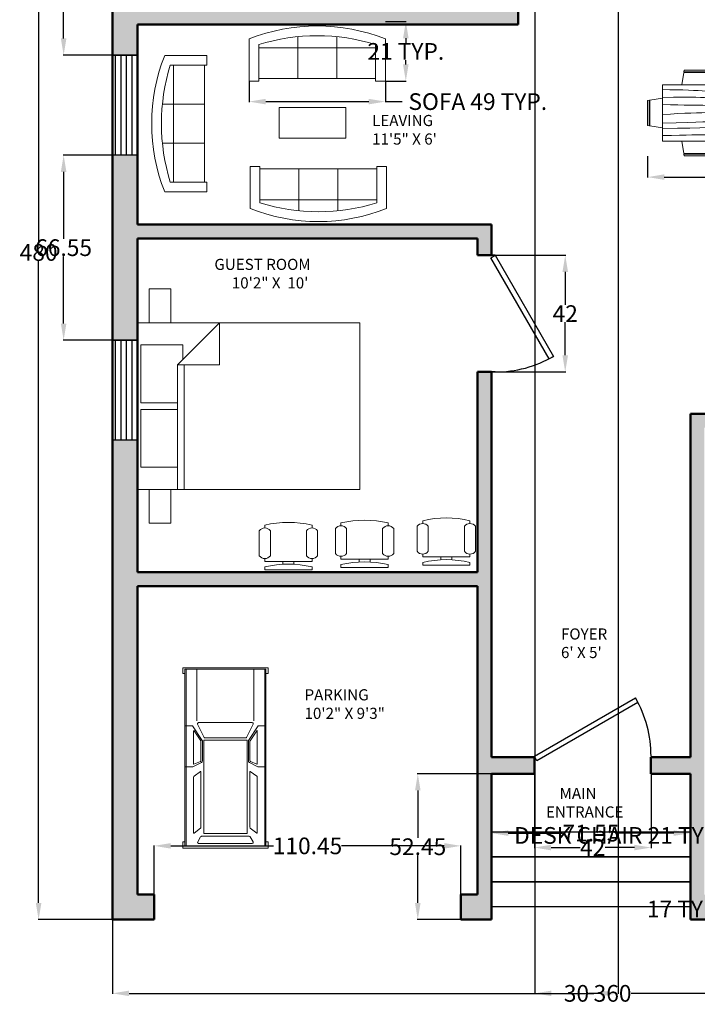
# Model space of a CAD drawing. Units: inches. Extents: x -40 to 482, y -490 to 102.
# Tile 1 of 4: x 2 to 245, y -490 to -136. Entities that reach past the tile are written whole.
import ezdxf

# ---------------------------------------------------------------- set-up
doc = ezdxf.new("R2010")
doc.units = ezdxf.units.IN
doc.header["$MEASUREMENT"] = 0
for name, color, linetype, lineweight in [('A-ANNO-DIMS', 2, 'Continuous', 18), ('A-ANNO-TEXT', 7, 'Continuous', 18), ('A-AREA-IDEN', 7, 'Continuous', 18), ('A-FLOR-PKNG', 8, 'Continuous', 13), ('A-FLOR-STRS', 7, 'Continuous', 25), ('A-FURN', 8, 'Continuous', 18), ('A-WALL', 7, 'Continuous', 50), ('A-WALL-PATT', 251, 'Continuous', 13), ('DOOR', 21, 'Continuous', 25), ('WINDOW', 151, 'Continuous', 25)]:
    doc.layers.add(name, color=color, linetype=linetype, lineweight=lineweight)
doc.styles.get("Standard").update_dxf_attribs({"font": 'arial.ttf'})
doc.dimstyles.get("Standard").update_dxf_attribs({"dimtxt": 6, "dimasz": 6, "dimexe": 0.18, "dimexo": 0.0625, "dimgap": 0.09, "dimtad": 0, "dimtih": 1, "dimtoh": 1, "dimdec": 3, "dimzin": 0, "dimdsep": 46, "dimlunit": 4, "dimtxsty": 'Standard', "dimcen": 0.09, "dimadec": 0, "dimazin": 0, "dimtfac": 1, "dimtdec": 3, "dimtofl": 0, "dimtmove": 0, "dimatfit": 3, "dimfxl": 1, "dimtolj": 1, "dimtzin": 0, "dimarcsym": 0})

# ---------------------------------------------------------------- blocks, each defined once
blk = doc.blocks.new('*U20')
for p, q in [((0, 0), (0, -6)), ((40, 0), (40, -6))]:
    blk.add_line(p, q)
blk.add_lwpolyline([(0, 0), (34.64, 20), (35.52, 18.48), (0.87, -1.52)], close=True)
blk.add_arc((0, 0), 40, 0, 30)
blk = doc.blocks.new('*U2')
for p, q in [((0, 0), (0, -6)), ((40, 0), (40, -6))]:
    blk.add_line(p, q)
blk.add_lwpolyline([(0, 0), (34.64, 20), (35.52, 18.48), (0.87, -1.52)], close=True)
blk.add_arc((0, 0), 40, 0, 30)
blk = doc.blocks.new('WINDOW')
for p, q in [((0, 0), (36, 0)), ((0, -9), (0, 0)), ((36, 0), (36, -9)), ((0, -2), (36, -2)), ((0, -4), (36, -4)), ((0, -6), (36, -6)), ((0, -8), (36, -8)), ((36, -9), (0, -9))]:
    blk.add_line(p, q)
blk = doc.blocks.new('Sofa - Roundback 7 ft.')
for p, q in [((-36.000027, -34), (-36.000027, -11.4696)), ((-12.00002, -32.4421), (-12.00003, -6.5971)), ((11.99997, -32.4421), (11.99998, -6.5971)), ((35.99998, -34), (35.99998, -11.4696)), ((-35.999844, -13.3819), (35.9998, -13.3819)), ((-36.000027, -32.4421), (35.99998, -32.4421))]:
    blk.add_line(p, q)
for points in [[(-36.000027, -34), (-42.000027, -34), (-42.000027, -8)], [(41.99998, -8), (41.99998, -34), (35.99998, -34)]]:
    blk.add_lwpolyline(points)
for centre, radius, start, end in [((0, -114.25), 114.25, 68.43141, 111.5686), ((-0.00001, -127.1968), 121.1968, 72.72033, 107.2797)]:
    blk.add_arc(centre, radius, start, end)
blk = doc.blocks.new('*U11')
for p, q in [((32, 987), (4462, 987)), ((32, 715), (1324, 715)), ((32, -715), (1324, -715)), ((32, -987), (4462, -987))]:
    blk.add_line(p, q)
for points in [[(141, 1016), (141, 1071), (0, 1071), (0, -1071), (141, -1071), (141, -1016), (32, -1016), (32, 1016)], [(32, 1016), (4462, 1016), (4462, -1016), (32, -1016)], [(4362, 1016), (4462, 1016), (4462, -1016), (4362, -1016), (4362, -1071), (4525, -1071), (4525, 1071), (4362, 1071)], [(1815, 546), (4151, 546), (4151, -546), (1815, -546)]]:
    blk.add_lwpolyline(points, close=True)
for points in [[(1451, 1016), (1451, 823), (1822, 580, 0.086577), (1843, 576), (2326, 576, 0.227875), (2376, 600), (2482, 816), (2482, 1016)], [(1451, -1016), (1451, -823), (1822, -580, -0.086577), (1843, -576), (2326, -576, -0.227875), (2376, -600), (2482, -816), (2482, -1016)]]:
    blk.add_lwpolyline(points, format="xyb")
for points in [[(1577, 786), (1832, 618, 0.146139), (1846, 614), (2322, 614, 0.29766), (2345, 629), (2415, 789, 0.541236), (2409, 798), (1580, 798, 0.744989)], [(2596, 624), (2717, 787, -0.236929), (2737, 798), (4138, 798, -0.621576), (4143, 787), (4018, 624, -0.233368), (3998, 614), (2601, 614, -0.616908)], [(1410, 697), (1742, 531, -0.284287), (1756, 508), (1756, -508, -0.284287), (1742, -531), (1410, -697, -0.557284), (1373, -674), (1373, 674, -0.557284)], [(4366, 694), (4237, 622, 0.271143), (4224, 599), (4224, -599, 0.271143), (4237, -622), (4366, -694, 0.573387), (4404, -672), (4404, 672, 0.573387)], [(1577, -786), (1832, -618, -0.146139), (1846, -614), (2322, -614, -0.29766), (2345, -629), (2415, -789, -0.541236), (2409, -798), (1580, -798, -0.744989)], [(2596, -624), (2717, -787, 0.236929), (2737, -798), (4138, -798, 0.621576), (4143, -787), (4018, -624, 0.233368), (3998, -614), (2601, -614, 0.616908)]]:
    blk.add_lwpolyline(points, format="xyb", close=True)
blk = doc.blocks.new('Bed - Queen')
for p, q in [((0, -80.00003), (0, 0)), ((0, 0), (59.99999, 0)), ((59.99999, 0), (59.99999, -80.00003)), ((7.99999, -1.2), (28.79998, -1.2)), ((7.99999, -14.4), (7.99999, -1.2)), ((28.79998, -1.2), (28.79998, -14.4)), ((31.19999, -1.2), (51.99999, -1.2)), ((31.19999, -14.4), (31.19999, -1.2)), ((51.99999, -1.2), (51.99999, -16.4)), ((0, -14.4), (44.8, -14.4)), ((44.8, -16.8), (0, -16.8)), ((59.99999, -29.6), (44.8, -14.4)), ((44.8, -14.4), (44.8, -29.6)), ((51.99999, -16.4), (46.79936, -16.4)), ((44.8, -29.6), (59.99999, -29.6)), ((59.99999, -80.00003), (0, -80.00003))]:
    blk.add_line(p, q)
blk = doc.blocks.new('Chair - Desk')
for p, q in [((-8.5, 0), (-8.5, -1)), ((-8.5, 0), (8.5, 0)), ((8.5, 0), (8.5, -1)), ((-8.5, -3), (-8.5, -4)), ((-8.5, -3), (8.5, -3)), ((-2, -3), (-2, -1.9355)), ((2, -1.9576), (2, -3)), ((8.5, -3), (8.5, -4)), ((-10.5, -5), (-10.5, -14)), ((-6.5, -14), (-6.5, -5)), ((6.5, -5), (6.5, -14)), ((10.5, -14), (10.5, -5)), ((-8.5, -15), (-8.5, -16)), ((8.5, -15), (8.5, -16))]:
    blk.add_line(p, q)
for centre, radius, start, end in [((0, 34.625), 36.625, 256.5803, 283.4197), ((-8.5, -6.5), 2.5, 36.8699, 143.1301), ((8.5, -6.5), 2.5, 36.8699, 143.1301), ((-8.5, -12.5), 2.5, 216.8699, 323.1301), ((8.5, -12.5), 2.5, 216.8699, 323.1301), ((0, 19.625), 36.625, 256.5803, 283.4197)]:
    blk.add_arc(centre, radius, start, end)
blk = doc.blocks.new('Dining Set - 36 x 72 in.')
for p, q in [((-22.2343, 26.00059), (-23.4847, 17.99762)), ((-22.2304, 26), (-5.7608, 26)), ((-22, 27.5), (-22.1562, 26.50042)), ((-5.8416, 26.5), (-22.1534, 26.5)), ((-22, 27.5), (-6, 27.5)), ((-5.8437, 26.49966), (-6, 27.5)), ((-4.5152, 17.99762), (-5.7655, 25.99926)), ((5.7657, 26.00059), (4.5153, 17.99762)), ((5.7696, 26), (22.2392, 26)), ((6, 27.5), (5.8438, 26.50042)), ((22.1584, 26.5), (5.8466, 26.5)), ((6, 27.5), (22, 27.5)), ((22.1563, 26.49966), (22, 27.5)), ((23.4848, 17.99762), (22.2345, 25.99926)), ((36, 18), (-36, 18)), ((-36, 18), (-36, -18)), ((36, -18), (36, 18)), ((-45.5, 8), (-44.5004, 8.15617)), ((-45.5, 8), (-45.5, -8)), ((-44.5, -8.15843), (-44.5, 8.15338)), ((-44.0006, 8.23428), (-35.9976, 9.48474)), ((-44, 8.23041), (-44, -8.23915)), ((44.0006, 8.23428), (35.9976, 9.48474)), ((44, 8.23041), (44, -8.23915)), ((44.5, -8.15843), (44.5, 8.15338)), ((45.5, 8), (44.5005, 8.15617)), ((45.5, 8), (45.5, -8)), ((-44.4997, -8.15631), (-45.5, -8)), ((-35.9976, -9.48476), (-43.9993, -8.2345)), ((35.9976, -9.48476), (43.9993, -8.2345)), ((44.4997, -8.15631), (45.5, -8)), ((-36, -18), (36, -18)), ((-22.2343, -26.0006), (-23.4847, -17.99762)), ((-4.5152, -17.99762), (-5.7655, -25.99928)), ((5.7657, -26.0006), (4.5153, -17.99762)), ((23.4848, -17.99762), (22.2345, -25.99928)), ((-22.2304, -26), (-5.7608, -26)), ((-22, -27.5), (-22.1562, -26.50044)), ((-5.8416, -26.5), (-22.1534, -26.5)), ((-22, -27.5), (-6, -27.5)), ((-5.8437, -26.49967), (-6, -27.5)), ((5.7696, -26), (22.2392, -26)), ((6, -27.5), (5.8438, -26.50044)), ((22.1584, -26.5), (5.8466, -26.5)), ((6, -27.5), (22, -27.5)), ((22.1563, -26.49967), (22, -27.5))]:
    blk.add_line(p, q)
for points in [[(-36, 15), (-31.1772, 14.97754), (-26.8079, 14.91406), (-22.8538, 14.81543), (-19.276, 14.6875), (-16.0362, 14.53613), (-13.0957, 14.36718), (-10.4159, 14.18652), (-7.9583, 14), (-5.6904, 13.81315), (-3.6035, 13.63021), (-1.6954, 13.45508), (0.0365, 13.29166), (1.5945, 13.14388), (2.9811, 13.01562), (4.1988, 12.9108), (5.25, 12.83333), (6.1393, 12.78613), (6.8802, 12.76823), (7.4883, 12.77767), (7.9792, 12.8125), (8.3685, 12.87077), (8.6719, 12.95052), (8.9049, 13.0498), (9.0833, 13.16666), (9.2205, 13.29899), (9.3216, 13.44401), (9.3895, 13.59879), (9.4271, 13.76041), (9.4373, 13.92594), (9.4232, 14.09245), (9.3875, 14.257), (9.3333, 14.41666), (9.2638, 14.56917), (9.1836, 14.71484), (9.0975, 14.85465), (9.0104, 14.98958), (8.9272, 15.1206), (8.8529, 15.2487), (8.7922, 15.37483), (8.75, 15.5), (8.7305, 15.62467), (8.7344, 15.74739), (8.7617, 15.86621), (8.8125, 15.97916), (8.8867, 16.08431), (8.9844, 16.17968), (9.1055, 16.26334), (9.25, 16.33333), (9.4189, 16.38802), (9.6172, 16.42708), (9.8506, 16.45052), (10.125, 16.45833), (10.4463, 16.45052), (10.8203, 16.42708), (11.2529, 16.38802), (11.75, 16.33333), (12.3184, 16.26318), (12.9694, 16.17838), (13.7151, 16.07991), (14.5677, 15.96875), (15.5395, 15.84586), (16.6426, 15.71224), (17.8893, 15.56884), (19.2917, 15.41666), (20.859, 15.25667), (22.5879, 15.08984), (24.4721, 14.91715), (26.5052, 14.73958), (28.6809, 14.5581), (30.9929, 14.3737), (33.4347, 14.18733), (36, 14)], [(-36, 10), (-28.9766, 10.14274), (-23.1725, 10.20442), (-18.4241, 10.19775), (-14.5677, 10.13541), (-11.4399, 10.03011), (-8.877, 9.89453), (-6.7154, 9.74137), (-4.7917, 9.58333), (-2.9698, 9.43082), (-1.2246, 9.28515), (0.4415, 9.14534), (2.026, 9.01041), (3.5266, 8.87939), (4.9408, 8.7513), (6.266, 8.62516), (7.5, 8.5), (8.6411, 8.37549), (9.6914, 8.2539), (10.6538, 8.13818), (11.5312, 8.03125), (12.3267, 7.93603), (13.043, 7.85547), (13.6831, 7.79248), (14.25, 7.75), (14.7471, 7.7303), (15.1797, 7.73307), (15.5537, 7.75732), (15.875, 7.80208), (16.1494, 7.86637), (16.3828, 7.94922), (16.5811, 8.04964), (16.75, 8.16666), (16.8944, 8.29915), (17.0143, 8.44531), (17.1089, 8.60319), (17.1771, 8.77083), (17.218, 8.94629), (17.2305, 9.1276), (17.2137, 9.31282), (17.1667, 9.5), (17.0895, 9.6875), (16.987, 9.875), (16.8649, 10.0625), (16.7292, 10.25), (16.5856, 10.4375), (16.4401, 10.625), (16.2985, 10.8125), (16.1667, 11), (16.05, 11.18733), (15.9518, 11.3737), (15.8752, 11.5581), (15.8229, 11.73958), (15.798, 11.91715), (15.8034, 12.08984), (15.842, 12.25667), (15.9167, 12.41666), (16.0295, 12.56836), (16.1784, 12.70833), (16.3605, 12.83268), (16.5729, 12.9375), (16.8127, 13.01888), (17.0768, 13.07291), (17.3625, 13.0957), (17.6667, 13.08333), (17.9894, 13.03312), (18.3418, 12.94726), (18.7382, 12.82918), (19.1927, 12.68229), (19.7195, 12.51001), (20.3327, 12.31575), (21.0465, 12.10294), (21.875, 11.875), (22.8357, 11.63354), (23.959, 11.37304), (25.2786, 11.08618), (26.8282, 10.76562), (28.6414, 10.40405), (30.752, 9.99414), (33.1936, 9.52856), (36, 9)], [(-36, 5.5), (-30.7157, 5.3348), (-26.069, 5.20963), (-21.9946, 5.11767), (-18.4271, 5.05208), (-15.3009, 5.00602), (-12.5508, 4.97265), (-10.1112, 4.94515), (-7.9167, 4.91666), (-5.909, 4.88167), (-4.0586, 4.83984), (-2.3429, 4.79215), (-0.7396, 4.73958), (0.7739, 4.6831), (2.22, 4.6237), (3.6213, 4.56233), (5, 4.5), (6.373, 4.43782), (7.7344, 4.3776), (9.0723, 4.32129), (10.375, 4.27083), (11.6309, 4.22819), (12.8281, 4.19531), (13.9551, 4.17415), (15, 4.16666), (15.954, 4.17448), (16.819, 4.19791), (17.6001, 4.23698), (18.3021, 4.29166), (18.9299, 4.36198), (19.4883, 4.44791), (19.9823, 4.54948), (20.4167, 4.66666), (20.7969, 4.79899), (21.1302, 4.94401), (21.4245, 5.09879), (21.6875, 5.26041), (21.9271, 5.42594), (22.1511, 5.59245), (22.3672, 5.757), (22.5834, 5.91666), (22.8065, 6.06868), (23.0404, 6.21093), (23.2879, 6.34147), (23.5521, 6.45833), (23.8358, 6.55957), (24.142, 6.64323), (24.4735, 6.70735), (24.8334, 6.75), (25.2235, 6.76969), (25.642, 6.76692), (26.0858, 6.74267), (26.5521, 6.69791), (27.0379, 6.63362), (27.5404, 6.55078), (28.0565, 6.45036), (28.5834, 6.33333), (29.1242, 6.19987), (29.7071, 6.04687), (30.3661, 5.87044), (31.1354, 5.66666), (32.0493, 5.43164), (33.142, 5.16146), (34.4475, 4.85221), (36, 4.5)], [(-36, -1), (-30.7915, -0.6591), (-26.0195, -0.38216), (-21.6519, -0.16284), (-17.6563, 0.00521), (-14.0005, 0.12833), (-10.6523, 0.21289), (-7.5796, 0.26522), (-4.75, 0.29166), (-2.134, 0.29793), (0.2878, 0.28711), (2.5317, 0.26163), (4.6146, 0.22396), (6.5529, 0.17651), (8.3633, 0.12174), (10.0623, 0.06209), (11.6667, 0), (13.1899, -0.06201), (14.6341, -0.1211), (15.9982, -0.17432), (17.2813, -0.21875), (18.4823, -0.25147), (19.6003, -0.26953), (20.6343, -0.27002), (21.5834, -0.25), (22.4481, -0.20768), (23.2357, -0.14584), (23.9549, -0.06836), (24.6146, 0.02083), (25.2235, 0.11784), (25.7904, 0.21875), (26.3241, 0.31966), (26.8334, 0.41666), (27.3265, 0.50618), (27.8099, 0.58593), (28.2894, 0.65397), (28.7709, 0.70833), (29.2601, 0.74707), (29.763, 0.76823), (30.2855, 0.76985), (30.8334, 0.75), (31.4088, 0.70784), (31.9994, 0.64713), (32.589, 0.57275), (33.1615, 0.48958), (33.7008, 0.4025), (34.1908, 0.3164), (34.6153, 0.23616), (34.9584, 0.16666), (35.2099, 0.11165), (35.3848, 0.07031), (35.504, 0.04069), (35.5886, 0.02083), (35.6594, 0.00879), (35.7377, 0.0026), (35.8442, 0.00032), (36, 0)], [(-36, -6.5), (-27.1843, -6.31267), (-20.084, -6.1263), (-14.469, -5.9419), (-10.1094, -5.76042), (-6.7752, -5.58285), (-4.2363, -5.41016), (-2.2629, -5.24333), (-0.625, -5.08334), (0.8708, -4.93099), (2.2715, -4.78646), (3.5872, -4.64974), (4.8281, -4.52084), (6.0046, -4.39974), (7.127, -4.28646), (8.2053, -4.18099), (9.25, -4.08334), (10.2705, -3.99382), (11.2734, -3.91407), (12.2647, -3.84603), (13.25, -3.79167), (14.2354, -3.75293), (15.2266, -3.73177), (16.2295, -3.73015), (17.25, -3.75), (18.2912, -3.79248), (19.3451, -3.85547), (20.4009, -3.93604), (21.4479, -4.03125), (22.4754, -4.13819), (23.4727, -4.25391), (24.4289, -4.37549), (25.3334, -4.5), (26.1785, -4.62492), (26.9694, -4.74935), (27.7145, -4.87281), (28.4219, -4.99479), (29.1, -5.11483), (29.7572, -5.23242), (30.4016, -5.34709), (31.0417, -5.45834), (31.6837, -5.56437), (32.3262, -5.65821), (32.9658, -5.73153), (33.599, -5.77604), (34.2224, -5.78345), (34.8327, -5.74545), (35.4264, -5.65373), (36, -5.5)], [(-36, -10), (-26.4022, -9.81299), (-18.4675, -9.62891), (-11.9839, -9.45069), (-6.7396, -9.28125), (-2.5226, -9.12354), (0.8789, -8.98047), (3.6769, -8.85498), (6.0833, -8.75), (8.2767, -8.66765), (10.3021, -8.60677), (12.1712, -8.56543), (13.8958, -8.54167), (15.4876, -8.53353), (16.9583, -8.53907), (18.3197, -8.55632), (19.5834, -8.58334), (20.7616, -8.61841), (21.8685, -8.66081), (22.9188, -8.71004), (23.9271, -8.76563), (24.9081, -8.82707), (25.8763, -8.89388), (26.8465, -8.96558), (27.8334, -9.04167), (28.8474, -9.12118), (29.8828, -9.20117), (30.93, -9.27824), (31.9792, -9.34896), (33.0205, -9.40991), (34.0443, -9.45768), (35.0407, -9.48885), (36, -9.5)], [(-36, -14.5), (-30.0881, -14.33513), (-25.0332, -14.21224), (-20.7312, -14.12647), (-17.0781, -14.07292), (-13.97, -14.04671), (-11.3027, -14.04297), (-8.9724, -14.05681), (-6.875, -14.08334), (-4.9224, -14.11833), (-3.0905, -14.16016), (-1.3709, -14.20785), (0.2448, -14.26042), (1.7647, -14.3169), (3.1973, -14.3763), (4.5507, -14.43767), (5.8333, -14.5), (7.0554, -14.5621), (8.235, -14.62175), (9.3922, -14.67652), (10.5469, -14.72396), (11.7192, -14.76164), (12.929, -14.78711), (14.1965, -14.79794), (15.5417, -14.79167), (16.9933, -14.76424), (18.6152, -14.70508), (20.4804, -14.60197), (22.6615, -14.44271), (25.2312, -14.21509), (28.2624, -13.9069), (31.8277, -13.50594), (36, -13)]]:
    blk.add_lwpolyline(points)
blk = doc.blocks.new('NIGHTSTAND')
blk.add_lwpolyline([(0, 12.15), (7.78, 12.15), (7.78, 0), (0, 0)], close=True)
blk = doc.blocks.new('*D28')
at = {"layer": 'A-ANNO-DIMS', "color": 0, "lineweight": -2, "transparency": 16777216}
for p, q in [((264.6, -429.23), (258.6, -429.23)), ((264.6, -432.32), (264.6, -429.05)), ((279.6, -429.23), (270.6, -429.23)), ((285.6, -432.32), (285.6, -429.05))]:
    blk.add_line(p, q, dxfattribs=at)
at = {"layer": 'A-ANNO-DIMS', "color": 0, "transparency": 16777216}
for points in [[(270.6, -428.23), (270.6, -430.23), (264.6, -429.23)], [(279.6, -428.23), (279.6, -430.23), (285.6, -429.23)]]:
    blk.add_solid(points, dxfattribs=at)
at = {"layer": 'Defpoints', "color": 0, "transparency": 16777216}
for p in [(264.6, -429.23), (264.6, -432.38), (285.6, -432.38)]:
    blk.add_point(p, dxfattribs=at)
at = {"layer": 'A-ANNO-DIMS', "color": 0, "transparency": 16777216, "insert": (217.27, -429.23), "char_height": 6, "attachment_point": 5}
blk.add_mtext('\\A1;DESK CHAIR 21 TYP.', dxfattribs=at)
blk = doc.blocks.new('*D29')
at = {"layer": 'A-ANNO-DIMS', "color": 0, "lineweight": -2, "transparency": 16777216}
for p, q in [((264.53, -432.38), (261.27, -432.38)), ((261.45, -438.38), (261.45, -443.71)), ((264.53, -449.71), (261.27, -449.71)), ((261.45, -449.71), (261.45, -455.71)), ((261.45, -455.71), (255.45, -455.71))]:
    blk.add_line(p, q, dxfattribs=at)
at = {"layer": 'A-ANNO-DIMS', "color": 0, "transparency": 16777216}
for points in [[(260.45, -438.38), (262.45, -438.38), (261.45, -432.38)], [(260.45, -443.71), (262.45, -443.71), (261.45, -449.71)]]:
    blk.add_solid(points, dxfattribs=at)
at = {"layer": 'Defpoints', "color": 0, "transparency": 16777216}
for p in [(264.6, -432.38), (261.45, -449.71), (264.6, -449.71)]:
    blk.add_point(p, dxfattribs=at)
at = {"layer": 'A-ANNO-DIMS', "color": 0, "transparency": 16777216, "insert": (241.04, -455.71), "char_height": 6, "attachment_point": 5}
blk.add_mtext('\\A1;17 TYP.', dxfattribs=at)
blk = doc.blocks.new('*D34')
at = {"layer": 'A-ANNO-DIMS', "color": 0, "lineweight": -2, "transparency": 16777216}
for p, q in [((84.04, -157.95), (84.04, -165.42)), ((133.1, -157.95), (133.1, -165.42)), ((90.04, -165.24), (127.1, -165.24)), ((133.1, -165.24), (139.1, -165.24))]:
    blk.add_line(p, q, dxfattribs=at)
at = {"layer": 'A-ANNO-DIMS', "color": 0, "transparency": 16777216}
for points in [[(90.04, -164.24), (90.04, -166.24), (84.04, -165.24)], [(127.1, -164.24), (127.1, -166.24), (133.1, -165.24)]]:
    blk.add_solid(points, dxfattribs=at)
at = {"layer": 'Defpoints', "color": 0, "transparency": 16777216}
for p in [(84.04, -157.88), (133.1, -157.88), (133.1, -165.24)]:
    blk.add_point(p, dxfattribs=at)
at = {"layer": 'A-ANNO-DIMS', "color": 0, "transparency": 16777216, "insert": (166.36, -165.24), "char_height": 6, "attachment_point": 5}
blk.add_mtext('\\A1;SOFA 49 TYP.', dxfattribs=at)
blk = doc.blocks.new('*D35')
at = {"layer": 'A-ANNO-DIMS', "color": 0, "lineweight": -2, "transparency": 16777216}
for p, q in [((133.17, -136.47), (140.64, -136.47)), ((140.46, -142.47), (140.46, -144.07)), ((140.46, -151.88), (140.46, -150.28)), ((133.17, -157.88), (140.64, -157.88))]:
    blk.add_line(p, q, dxfattribs=at)
at = {"layer": 'A-ANNO-DIMS', "color": 0, "transparency": 16777216}
for points in [[(139.46, -142.47), (141.46, -142.47), (140.46, -136.47)], [(139.46, -151.88), (141.46, -151.88), (140.46, -157.88)]]:
    blk.add_solid(points, dxfattribs=at)
at = {"layer": 'Defpoints', "color": 0, "transparency": 16777216}
for p in [(133.1, -136.47), (140.46, -136.47), (133.1, -157.88)]:
    blk.add_point(p, dxfattribs=at)
at = {"layer": 'A-ANNO-DIMS', "color": 0, "transparency": 16777216, "insert": (140.46, -147.18), "char_height": 6, "attachment_point": 5}
blk.add_mtext('\\A1;21 TYP.', dxfattribs=at)
blk = doc.blocks.new('*D50')
at = {"layer": 'A-ANNO-DIMS', "color": 0, "lineweight": -2, "transparency": 16777216}
for p, q in [((227.47, -184.82), (227.47, -192.58)), ((278.45, -184.82), (278.45, -192.58)), ((233.47, -192.4), (272.45, -192.4)), ((278.45, -192.4), (284.45, -192.4))]:
    blk.add_line(p, q, dxfattribs=at)
at = {"layer": 'A-ANNO-DIMS', "color": 0, "transparency": 16777216}
for points in [[(233.47, -191.4), (233.47, -193.4), (227.47, -192.4)], [(272.45, -191.4), (272.45, -193.4), (278.45, -192.4)]]:
    blk.add_solid(points, dxfattribs=at)
at = {"layer": 'Defpoints', "color": 0, "transparency": 16777216}
for p in [(227.47, -184.75), (278.45, -184.75), (278.45, -192.4)]:
    blk.add_point(p, dxfattribs=at)
at = {"layer": 'A-ANNO-DIMS', "color": 0, "transparency": 16777216, "insert": (313.26, -192.4), "char_height": 6, "attachment_point": 5}
blk.add_mtext('\\A1;DINING SET 51', dxfattribs=at)
blk = doc.blocks.new('*D52')
at = {"layer": 'A-ANNO-DIMS', "color": 0, "lineweight": -2, "transparency": 16777216}
for p, q in [((34.86, -459.57), (34.86, -486.22)), ((394.86, -459.57), (394.86, -486.22)), ((40.86, -486.04), (208.15, -486.04)), ((388.86, -486.04), (221.56, -486.04))]:
    blk.add_line(p, q, dxfattribs=at)
at = {"layer": 'A-ANNO-DIMS', "color": 0, "transparency": 16777216}
for points in [[(40.86, -485.04), (40.86, -487.04), (34.86, -486.04)], [(388.86, -485.04), (388.86, -487.04), (394.86, -486.04)]]:
    blk.add_solid(points, dxfattribs=at)
at = {"layer": 'Defpoints', "color": 0, "transparency": 16777216}
for p in [(34.86, -459.51), (394.86, -459.51), (394.86, -486.04)]:
    blk.add_point(p, dxfattribs=at)
at = {"layer": 'A-ANNO-DIMS', "color": 0, "transparency": 16777216, "insert": (214.86, -486.04), "char_height": 6, "attachment_point": 5}
blk.add_mtext('\\A1;360', dxfattribs=at)
blk = doc.blocks.new('*D53')
at = {"layer": 'A-ANNO-DIMS', "color": 0, "lineweight": -2, "transparency": 16777216}
for p, q in [((34.79, 20.49), (8.14, 20.49)), ((8.32, 14.49), (8.32, -216.36)), ((8.32, -453.51), (8.32, -222.66)), ((34.79, -459.51), (8.14, -459.51))]:
    blk.add_line(p, q, dxfattribs=at)
at = {"layer": 'A-ANNO-DIMS', "color": 0, "transparency": 16777216}
for points in [[(7.32, 14.49), (9.32, 14.49), (8.32, 20.49)], [(7.32, -453.51), (9.32, -453.51), (8.32, -459.51)]]:
    blk.add_solid(points, dxfattribs=at)
at = {"layer": 'Defpoints', "color": 0, "transparency": 16777216}
for p in [(8.32, 20.49), (34.86, 20.49), (34.86, -459.51)]:
    blk.add_point(p, dxfattribs=at)
at = {"layer": 'A-ANNO-DIMS', "color": 0, "transparency": 16777216, "insert": (8.32, -219.51), "char_height": 6, "attachment_point": 5}
blk.add_mtext('\\A1;480', dxfattribs=at)
blk = doc.blocks.new('*D57')
at = {"layer": 'A-ANNO-DIMS', "color": 0, "lineweight": -2, "transparency": 16777216}
for p, q in [((43.79, -76.86), (17.14, -76.86)), ((17.32, -82.86), (17.32, -109.54)), ((17.32, -142.52), (17.32, -115.84)), ((43.79, -148.52), (17.14, -148.52))]:
    blk.add_line(p, q, dxfattribs=at)
at = {"layer": 'A-ANNO-DIMS', "color": 0, "transparency": 16777216}
for points in [[(16.32, -82.86), (18.32, -82.86), (17.32, -76.86)], [(16.32, -142.52), (18.32, -142.52), (17.32, -148.52)]]:
    blk.add_solid(points, dxfattribs=at)
at = {"layer": 'Defpoints', "color": 0, "transparency": 16777216}
for p in [(17.32, -76.86), (43.86, -76.86), (43.86, -148.52)]:
    blk.add_point(p, dxfattribs=at)
at = {"layer": 'A-ANNO-DIMS', "color": 0, "transparency": 16777216, "insert": (17.32, -112.69), "char_height": 6, "attachment_point": 5}
blk.add_mtext('\\A1;71.66', dxfattribs=at)
blk = doc.blocks.new('*D58')
at = {"layer": 'A-ANNO-DIMS', "color": 0, "lineweight": -2, "transparency": 16777216}
for p, q in [((43.79, -184.52), (17.14, -184.52)), ((17.32, -190.52), (17.32, -214.64)), ((17.32, -245.07), (17.32, -220.95)), ((43.79, -251.07), (17.14, -251.07))]:
    blk.add_line(p, q, dxfattribs=at)
at = {"layer": 'A-ANNO-DIMS', "color": 0, "transparency": 16777216}
for points in [[(16.32, -190.52), (18.32, -190.52), (17.32, -184.52)], [(16.32, -245.07), (18.32, -245.07), (17.32, -251.07)]]:
    blk.add_solid(points, dxfattribs=at)
at = {"layer": 'Defpoints', "color": 0, "transparency": 16777216}
for p in [(17.32, -184.52), (43.86, -184.52), (43.86, -251.07)]:
    blk.add_point(p, dxfattribs=at)
at = {"layer": 'A-ANNO-DIMS', "color": 0, "transparency": 16777216, "insert": (17.32, -217.79), "char_height": 6, "attachment_point": 5}
blk.add_mtext('\\A1;66.55', dxfattribs=at)
blk = doc.blocks.new('*D63')
at = {"layer": 'A-ANNO-DIMS', "color": 0, "lineweight": -2, "transparency": 16777216}
for p, q in [((186.86, -53.57), (186.86, -486.22)), ((216.86, -53.57), (216.86, -486.22)), ((192.86, -486.04), (197.48, -486.04)), ((210.86, -486.04), (206.23, -486.04))]:
    blk.add_line(p, q, dxfattribs=at)
at = {"layer": 'A-ANNO-DIMS', "color": 0, "transparency": 16777216}
for points in [[(192.86, -485.04), (192.86, -487.04), (186.86, -486.04)], [(210.86, -485.04), (210.86, -487.04), (216.86, -486.04)]]:
    blk.add_solid(points, dxfattribs=at)
at = {"layer": 'Defpoints', "color": 0, "transparency": 16777216}
for p in [(186.86, -53.51), (216.86, -53.51), (216.86, -486.04)]:
    blk.add_point(p, dxfattribs=at)
at = {"layer": 'A-ANNO-DIMS', "color": 0, "transparency": 16777216, "insert": (201.86, -486.04), "char_height": 6, "attachment_point": 5}
blk.add_mtext('\\A1;30', dxfattribs=at)
blk = doc.blocks.new('*D65')
at = {"layer": 'A-ANNO-DIMS', "color": 0, "lineweight": -2, "transparency": 16777216}
for p, q in [((171.36, -220.51), (198.01, -220.51)), ((197.83, -226.51), (197.83, -238.41)), ((197.83, -256.51), (197.83, -244.61)), ((171.36, -262.51), (198.01, -262.51))]:
    blk.add_line(p, q, dxfattribs=at)
at = {"layer": 'A-ANNO-DIMS', "color": 0, "transparency": 16777216}
for points in [[(196.83, -226.51), (198.83, -226.51), (197.83, -220.51)], [(196.83, -256.51), (198.83, -256.51), (197.83, -262.51)]]:
    blk.add_solid(points, dxfattribs=at)
at = {"layer": 'Defpoints', "color": 0, "transparency": 16777216}
for p in [(171.3, -220.51), (171.3, -262.51), (197.83, -262.51)]:
    blk.add_point(p, dxfattribs=at)
at = {"layer": 'A-ANNO-DIMS', "color": 0, "transparency": 16777216, "insert": (197.83, -241.51), "char_height": 6, "attachment_point": 5}
blk.add_mtext('\\A1;42', dxfattribs=at)
blk = doc.blocks.new('*D71')
at = {"layer": 'A-ANNO-DIMS', "color": 0, "lineweight": -2, "transparency": 16777216}
for p, q in [((49.86, -459.45), (49.86, -432.8)), ((55.86, -432.98), (92.79, -432.98)), ((154.3, -432.98), (117.36, -432.98)), ((160.3, -459.45), (160.3, -432.8))]:
    blk.add_line(p, q, dxfattribs=at)
at = {"layer": 'A-ANNO-DIMS', "color": 0, "transparency": 16777216}
for points in [[(55.86, -431.98), (55.86, -433.98), (49.86, -432.98)], [(154.3, -431.98), (154.3, -433.98), (160.3, -432.98)]]:
    blk.add_solid(points, dxfattribs=at)
at = {"layer": 'Defpoints', "color": 0, "transparency": 16777216}
for p in [(160.3, -432.98), (49.86, -459.51), (160.3, -459.51)]:
    blk.add_point(p, dxfattribs=at)
at = {"layer": 'A-ANNO-DIMS', "color": 0, "transparency": 16777216, "insert": (105.08, -432.98), "char_height": 6, "attachment_point": 5}
blk.add_mtext('\\A1;110.45', dxfattribs=at)
blk = doc.blocks.new('*D72')
at = {"layer": 'A-ANNO-DIMS', "color": 0, "lineweight": -2, "transparency": 16777216}
for p, q in [((171.3, -454.84), (171.3, -428.2)), ((177.3, -428.38), (196.87, -428.38)), ((236.86, -428.38), (217.29, -428.38)), ((242.86, -454.84), (242.86, -428.2))]:
    blk.add_line(p, q, dxfattribs=at)
at = {"layer": 'A-ANNO-DIMS', "color": 0, "transparency": 16777216}
for points in [[(177.3, -427.38), (177.3, -429.38), (171.3, -428.38)], [(236.86, -427.38), (236.86, -429.38), (242.86, -428.38)]]:
    blk.add_solid(points, dxfattribs=at)
at = {"layer": 'Defpoints', "color": 0, "transparency": 16777216}
for p in [(242.86, -428.38), (171.3, -454.91), (242.86, -454.91)]:
    blk.add_point(p, dxfattribs=at)
at = {"layer": 'A-ANNO-DIMS', "color": 0, "transparency": 16777216, "insert": (207.08, -428.38), "char_height": 6, "attachment_point": 5}
blk.add_mtext('\\A1;71.55', dxfattribs=at)
blk = doc.blocks.new('*D76')
at = {"layer": 'A-ANNO-DIMS', "color": 0, "lineweight": -2, "transparency": 16777216}
for p, q in [((186.71, -407.13), (186.71, -433.77)), ((228.71, -407.13), (228.71, -433.77)), ((192.71, -433.59), (203.23, -433.59)), ((222.71, -433.59), (212.19, -433.59))]:
    blk.add_line(p, q, dxfattribs=at)
at = {"layer": 'A-ANNO-DIMS', "color": 0, "transparency": 16777216}
for points in [[(192.71, -432.59), (192.71, -434.59), (186.71, -433.59)], [(222.71, -432.59), (222.71, -434.59), (228.71, -433.59)]]:
    blk.add_solid(points, dxfattribs=at)
at = {"layer": 'Defpoints', "color": 0, "transparency": 16777216}
for p in [(186.71, -407.06), (228.71, -407.06), (186.71, -433.59)]:
    blk.add_point(p, dxfattribs=at)
at = {"layer": 'A-ANNO-DIMS', "color": 0, "transparency": 16777216, "insert": (207.71, -433.59), "char_height": 6, "attachment_point": 5}
blk.add_mtext('\\A1;42', dxfattribs=at)
blk = doc.blocks.new('*D79')
at = {"layer": 'A-ANNO-DIMS', "color": 0, "lineweight": -2, "transparency": 16777216}
for p, q in [((171.24, -407.06), (144.59, -407.06)), ((144.77, -413.06), (144.77, -430.13)), ((144.77, -453.51), (144.77, -436.44)), ((171.24, -459.51), (144.59, -459.51))]:
    blk.add_line(p, q, dxfattribs=at)
at = {"layer": 'A-ANNO-DIMS', "color": 0, "transparency": 16777216}
for points in [[(143.77, -413.06), (145.77, -413.06), (144.77, -407.06)], [(143.77, -453.51), (145.77, -453.51), (144.77, -459.51)]]:
    blk.add_solid(points, dxfattribs=at)
at = {"layer": 'Defpoints', "color": 0, "transparency": 16777216}
for p in [(144.77, -407.06), (171.3, -407.06), (171.3, -459.51)]:
    blk.add_point(p, dxfattribs=at)
at = {"layer": 'A-ANNO-DIMS', "color": 0, "transparency": 16777216, "insert": (144.77, -433.29), "char_height": 6, "attachment_point": 5}
blk.add_mtext('\\A1;52.45', dxfattribs=at)

msp = doc.modelspace()

# ---------------------------------------------------------------- hatches: boundary and pattern name
at = {"layer": 'A-WALL-PATT'}
h = msp.add_hatch(color=256, dxfattribs=at)
h.dxf.hatch_style = 1
h.paths.add_polyline_path([(394.8554, -267.0722), (385.8554, -267.0722), (385.8554, -280.5091), (361.8554, -280.5091), (361.8554, -285.5091), (385.8554, -285.5091), (385.8554, -344.9426), (394.8554, -344.9426)])
h.paths.add_polyline_path([(394.8554, -171.3545), (385.8554, -171.3545), (385.8554, -185.5091), (325.8554, -185.5091), (325.8554, -173.5091), (320.8554, -173.5091), (320.8554, -190.5091), (320.8554, -277.5091), (295.8554, -277.5091), (295.8554, -282.5091), (320.8554, -282.5091), (320.8554, -285.5091), (331.8554, -285.5091), (331.8554, -280.5091), (325.8554, -280.5091), (325.8554, -190.5091), (386.1154, -190.5091), (386.1154, -226.6962), (386.0363, -243.0722), (394.8554, -243.0722)])
h.paths.add_polyline_path([(394.8554, -83.9679), (385.8554, -83.9679), (385.8554, -127.5091), (320.8554, -127.5091), (320.8554, -137.5091), (320.8554, -143.5091), (325.8554, -143.5091), (325.8554, -137.5091), (385.8554, -137.5091), (385.8554, -147.3545), (394.8554, -147.3545)])
h.paths.add_polyline_path([(394.8554, 20.4909), (235.3658, 20.4909), (235.3658, 11.4909), (270.8554, 11.4909), (270.9798, 11.1006), (270.9798, 3.1006), (270.8554, -48.5091), (216.8554, -48.5091), (216.8554, -53.5091), (270.8554, -53.5091), (270.8554, -132.5091), (275.8554, -132.5091), (275.8554, 11.4909), (311.8554, 11.4909), (385.8554, 11.4909), (385.8554, -47.9679), (394.8554, -47.9679)])
h.paths.add_polyline_path([(211.3658, 20.4909), (126.5194, 20.4909), (126.5194, 11.4909), (175.8554, 11.4909), (175.8554, -84.5091), (180.8554, -84.5091), (180.8554, -53.5091), (186.8554, -53.5091), (186.8554, -48.5091), (180.8554, -48.5091), (180.8554, 11.4909), (211.3658, 11.4909)])
h.paths.add_polyline_path([(90.5194, 20.4909), (34.8554, 20.4909), (34.8554, -40.8616), (43.8554, -40.8616), (43.8554, -28.8616), (43.8554, 11.4909), (90.5194, 11.4909)])
h.paths.add_polyline_path([(43.8554, -76.8616), (34.8554, -76.8616), (34.8554, -148.5194), (43.8554, -148.5194), (43.8554, -137.5091), (180.8554, -137.5091), (180.8554, -126.5091), (175.8554, -126.5091), (175.8554, -132.5091), (43.8554, -132.5091)])
h.paths.add_polyline_path([(171.3012, -209.5091), (43.8554, -209.5091), (43.8554, -184.5194), (34.8554, -184.5194), (34.8554, -251.068), (43.8554, -251.068), (43.8554, -244.7708), (43.8554, -214.5091), (166.3012, -214.5091), (166.3012, -220.5091), (171.3012, -220.5091)])
h.paths.add_polyline_path([(171.3012, -262.5091), (166.3012, -262.5091), (166.3012, -334.5091), (43.8554, -334.5091), (43.8554, -287.068), (34.8554, -287.068), (34.8554, -459.5091), (43.8554, -459.5091), (49.8554, -459.5091), (49.8554, -450.5091), (43.8554, -450.5091), (43.8554, -339.5091), (166.3012, -339.5091), (166.3012, -450.5091), (160.3012, -450.5091), (160.3012, -459.5091), (166.3012, -459.5091), (171.3012, -459.5091), (171.3012, -450.5091), (171.3012, -445.9382), (171.3012, -410.0635), (171.3012, -407.0635), (186.7114, -407.0635), (186.7114, -401.0635), (171.3012, -401.0635)])
h.paths.add_polyline_path([(394.8554, -380.9426), (385.8554, -380.9426), (385.8554, -450.5091), (247.8554, -450.5091), (247.8554, -282.5091), (253.8554, -282.5091), (253.8554, -277.5091), (242.8554, -277.5091), (242.8554, -401.0635), (228.7114, -401.0635), (228.7114, -407.0635), (242.8554, -407.0635), (242.8554, -410.0635), (242.8554, -419.0322), (242.8554, -450.5091), (242.8554, -454.9068), (242.8554, -459.5091), (394.8554, -459.5091)])

# ---------------------------------------------------------------- linework, layer by layer
at = {"layer": 'A-FLOR-STRS'}
for p, q in [((171.3012, -419.0322), (171.3012, -410.0635)), ((242.8554, -410.0635), (242.8554, -419.0322)), ((171.3012, -428.0008), (171.3012, -419.0322)), ((242.8554, -419.0322), (242.8554, -428.0008)), ((242.8554, -428.0008), (171.3012, -428.0008)), ((171.3012, -436.9695), (171.3012, -428.0008)), ((242.8554, -428.0008), (242.8554, -436.9695)), ((242.8554, -436.9695), (171.3012, -436.9695)), ((171.3012, -436.9695), (242.8554, -436.9695)), ((171.3012, -445.9382), (171.3012, -436.9695)), ((242.8554, -436.9695), (242.8554, -445.9382)), ((242.8554, -445.9382), (171.3012, -445.9382)), ((171.3012, -445.9382), (242.8554, -445.9382)), ((171.3012, -454.9068), (171.3012, -445.9382)), ((242.8554, -445.9382), (242.8554, -454.9068)), ((242.8554, -454.9068), (171.3012, -454.9068))]:
    msp.add_line(p, q, dxfattribs=at)
at = {"layer": 'A-FURN'}
msp.add_lwpolyline([(94.9274, -167.3616), (118.9274, -167.3616), (118.9274, -178.3616), (94.9274, -178.3616)], close=True, dxfattribs=at)
at = {"layer": 'A-WALL'}
for p, q in [((180.8554, -137.5091), (180.8554, -126.5091)), ((43.8554, -137.5091), (180.8554, -137.5091)), ((43.8554, -209.5091), (43.8554, -137.5091)), ((43.8554, -209.5091), (171.3012, -209.5091)), ((171.3012, -220.5091), (171.3012, -209.5091)), ((43.8554, -214.5091), (166.3012, -214.5091)), ((43.8554, -334.5091), (43.8554, -214.5091)), ((166.3012, -220.5091), (166.3012, -214.5091)), ((166.3012, -220.5091), (171.3012, -220.5091)), ((166.3012, -334.5091), (166.3012, -262.5091)), ((166.3012, -262.5091), (171.3012, -262.5091)), ((171.3012, -401.0635), (171.3012, -262.5091)), ((242.8554, -277.5091), (242.8554, -401.0635)), ((253.8554, -277.5091), (242.8554, -277.5091)), ((43.8554, -334.5091), (166.3012, -334.5091)), ((43.8554, -450.5091), (43.8554, -339.5091)), ((43.8554, -339.5091), (166.3012, -339.5091)), ((166.3012, -450.5091), (166.3012, -339.5091)), ((186.7114, -401.0635), (171.3012, -401.0635)), ((186.7114, -407.0635), (186.7114, -401.0635)), ((242.8554, -401.0635), (228.6245, -401.0635)), ((228.6245, -401.0635), (228.6245, -407.0635)), ((186.7114, -407.0635), (171.3012, -407.0635)), ((171.3012, -407.0635), (171.3012, -410.0635)), ((242.8554, -407.0635), (228.6245, -407.0635)), ((242.8554, -407.0635), (242.8554, -410.0635)), ((171.3012, -450.5091), (171.3012, -410.0635)), ((242.8554, -410.0635), (242.8554, -450.5091)), ((49.8554, -450.5091), (43.8554, -450.5091)), ((49.8554, -459.5091), (49.8554, -450.5091)), ((160.3012, -459.5091), (160.3012, -450.5091)), ((160.3012, -450.5091), (166.3012, -450.5091)), ((171.3012, -450.5091), (171.3012, -459.5091)), ((242.8554, -450.5091), (242.8554, -459.5091)), ((43.8554, -459.5091), (49.8554, -459.5091)), ((166.3012, -459.5091), (160.3012, -459.5091))]:
    msp.add_line(p, q, dxfattribs=at)
for points in [[(43.8554, -459.5091), (34.8554, -459.5091), (34.8554, 20.4909), (394.8554, 20.4909), (394.8554, -459.5091), (242.8554, -459.5091)], [(171.3012, -459.5091), (166.3012, -459.5091)]]:
    msp.add_lwpolyline(points, dxfattribs=at)

# ---------------------------------------------------------------- block references
at = {"layer": 'A-FLOR-PKNG', "xscale": 0.0143404532614813, "yscale": 0.0143404532614813, "zscale": 0.0143404532614813, "rotation": 270}
msp.add_blockref('*U11', (75.5482, -368.9608), dxfattribs=at)
at = {"layer": 'A-FURN'}
for name, p, xscale, yscale, zscale in [('Sofa - Roundback 7 ft.', (108.5719, -138.0262), 0.5840680911338632, 0.5840680911338632, 0.5840680911338632), ('Dining Set - 36 x 72 in.', (252.9608, -169.3451), 0.5602730891247094, 0.5602730891247094, 0.5602730891247094)]:
    msp.add_blockref(name, p, dxfattribs=dict(at, xscale=xscale, yscale=yscale, zscale=zscale))
at = {"layer": 'A-FURN', "xscale": 0.5840680911338632, "yscale": 0.5840680911338632, "zscale": 0.5840680911338632}
for p, rotation in [((49.011, -173.1518), 90), ((109.0044, -208.3865), 180)]:
    msp.add_blockref('Sofa - Roundback 7 ft.', p, dxfattribs=dict(at, rotation=rotation))
at = {"layer": 'A-FURN'}
for p in [(48.126, -244.7712), (48.126, -316.925)]:
    msp.add_blockref('NIGHTSTAND', p, dxfattribs=at)
for name, p, rotation in [('Bed - Queen', (43.8554, -304.7708), 90), ('Chair - Desk', (155.029, -332.0141), 180), ('Chair - Desk', (98.2162, -333.6238), 180), ('Chair - Desk', (125.6153, -332.819), 180)]:
    msp.add_blockref(name, p, dxfattribs=dict(at, rotation=rotation))
at = {"layer": 'DOOR', "xscale": 1.05, "yscale": 1.05, "zscale": 1.05, "rotation": 270}
msp.add_blockref('*U2', (172.6012, -220.5091), dxfattribs=at)
at = {"layer": 'DOOR', "xscale": 1.05, "yscale": 1.05, "zscale": 1.05}
msp.add_blockref('*U20', (186.7114, -400.7635), dxfattribs=at)
at = {"layer": 'WINDOW', "rotation": 270}
for p in [(43.8554, -148.5194), (43.8554, -251.068)]:
    msp.add_blockref('WINDOW', p, dxfattribs=at)

# ---------------------------------------------------------------- texts
at = {"layer": 'A-ANNO-TEXT', "insert": (190.9094, -412.1127), "char_height": 4, "attachment_point": 1}
msp.add_mtext_dynamic_manual_height_columns('    MAIN \\PENTRANCE', width=60.434946, gutter_width=1, heights=[0], dxfattribs=at)
at = {"layer": 'A-AREA-IDEN', "char_height": 4, "attachment_point": 1}
for s, width, insert in [('LEAVING\\P11\'5" X 6\'', 43.408776, (128.3275, -170.0403)), ('\\pxql;                GUEST ROOM   \\P\\pqc;10\'2" X  10\'', 79.218438, (52.0143, -221.792)), ("FOYER\\P6' X 5'", 56.795929, (196.2932, -354.7594)), ('PARKING\\P10\'2" X 9\'3"', 57.324243, (104.0086, -376.6342))]:
    msp.add_mtext_dynamic_manual_height_columns(s, width=width, gutter_width=1, heights=[0], dxfattribs=dict(at, insert=insert))

# ---------------------------------------------------------------- dimensions: what is measured, and where the dimension line sits
at = {"layer": 'A-ANNO-DIMS'}
for base, p1, p2, angle, override, picture, middle in [((8.3239, 20.4909), (34.8554, -459.5091), (34.8554, 20.4909), 90, {"dimdec": 0, "dimlfac": 1, "dimrnd": 0, "dimzin": 0, "dimdsep": 46, "dimlunit": 2}, '*D53', (8.3239, -219.5091)), ((17.3239, -76.8616), (43.8554, -148.5194), (43.8554, -76.8616), 90, {"dimdec": 2, "dimlfac": 1, "dimrnd": 0, "dimzin": 0, "dimdsep": 46, "dimlunit": 2}, '*D57', (17.3239, -112.6905)), ((17.3239, -184.5194), (43.8554, -251.068), (43.8554, -184.5194), 90, {"dimdec": 2, "dimlfac": 1, "dimrnd": 0, "dimzin": 0, "dimdsep": 46, "dimlunit": 2}, '*D58', (17.3239, -217.7937)), ((197.8327, -262.5091), (171.3012, -220.5091), (171.3012, -262.5091), 270, {"dimdec": 0, "dimlfac": 1, "dimrnd": 0, "dimzin": 0, "dimdsep": 46, "dimlunit": 2}, '*D65', (197.8327, -241.5091)), ((144.7697, -407.0635), (171.3012, -459.5091), (171.3012, -407.0635), 90, {"dimdec": 2, "dimlfac": 1, "dimrnd": 0, "dimzin": 0, "dimdsep": 46, "dimlunit": 2}, '*D79', (144.7697, -433.2863)), ((186.7114, -433.595), (228.7114, -407.0635), (186.7114, -407.0635), 180, {"dimdec": 0, "dimlfac": 1, "dimrnd": 0, "dimzin": 0, "dimdsep": 46, "dimlunit": 2}, '*D76', (207.7114, -433.595))]:
    dim = msp.add_linear_dim(base=base, p1=p1, p2=p2, angle=angle, dimstyle='Standard', override=override, dxfattribs=at)
    dim.commit()
    dim.dimension.update_dxf_attribs({"geometry": picture, "text_midpoint": middle})
for base, p1, p2, override, picture, middle in [((216.8554, -486.0406), (186.8554, -53.5091), (216.8554, -53.5091), {"dimdec": 0, "dimlfac": 1, "dimrnd": 0, "dimzin": 0, "dimdsep": 46, "dimlunit": 2}, '*D63', (201.8554, -486.0406)), ((242.8554, -428.3753), (171.3012, -454.9068), (242.8554, -454.9068), {"dimdec": 2, "dimlfac": 1, "dimrnd": 0, "dimzin": 0, "dimdsep": 46, "dimlunit": 2}, '*D72', (207.0783, -428.3753)), ((160.3012, -432.9776), (49.8554, -459.5091), (160.3012, -459.5091), {"dimdec": 2, "dimlfac": 1, "dimrnd": 0, "dimzin": 0, "dimdsep": 46, "dimlunit": 2}, '*D71', (105.0783, -432.9776)), ((394.8554, -486.0406), (34.8554, -459.5091), (394.8554, -459.5091), {"dimdec": 0, "dimlfac": 1, "dimrnd": 0, "dimzin": 0, "dimdsep": 46, "dimlunit": 2}, '*D52', (214.8554, -486.0406))]:
    dim = msp.add_linear_dim(base=base, p1=p1, p2=p2, dimstyle='Standard', override=override, dxfattribs=at)
    dim.commit()
    dim.dimension.update_dxf_attribs({"geometry": picture, "text_midpoint": middle})
for base, p1, p2, angle, text, picture, middle in [((140.462, -136.4687), (133.1028, -157.8845), (133.1028, -136.4687), 90, '<> TYP.', '*D35', (140.462, -147.1766)), ((264.5957, -429.2292), (285.5957, -432.3792), (264.5957, -432.3792), 180, 'DESK CHAIR <> TYP.', '*D28', (217.271, -429.2292)), ((261.4457, -449.7125), (264.5957, -432.3792), (264.5957, -449.7125), 270, '<> TYP.', '*D29', (241.0351, -455.7125))]:
    dim = msp.add_linear_dim(base=base, p1=p1, p2=p2, angle=angle, text=text, dimstyle='Standard', override={"dimdec": 0, "dimlfac": 1, "dimrnd": 0, "dimzin": 0, "dimdsep": 46, "dimlunit": 2}, dxfattribs=at)
    dim.commit()
    dim.dimension.update_dxf_attribs({"geometry": picture, "text_midpoint": middle})
for base, p1, p2, text, picture, middle in [((133.1028, -165.2438), (84.041, -157.8845), (133.1028, -157.8845), 'SOFA <> TYP.', '*D34', (166.3565, -165.2438)), ((278.4532, -192.4003), (227.4684, -184.7526), (278.4532, -184.7526), 'DINING SET <>', '*D50', (313.2601, -192.4003))]:
    dim = msp.add_linear_dim(base=base, p1=p1, p2=p2, text=text, dimstyle='Standard', override={"dimdec": 0, "dimlfac": 1, "dimrnd": 0, "dimzin": 0, "dimdsep": 46, "dimlunit": 2}, dxfattribs=at)
    dim.commit()
    dim.dimension.update_dxf_attribs({"geometry": picture, "text_midpoint": middle})

doc.saveas('drawing.dxf')
